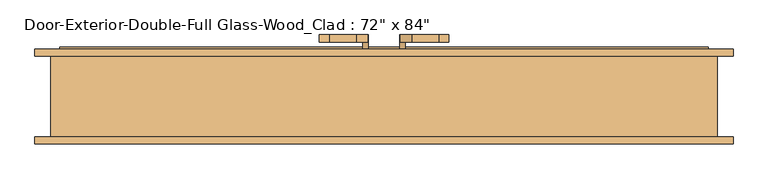
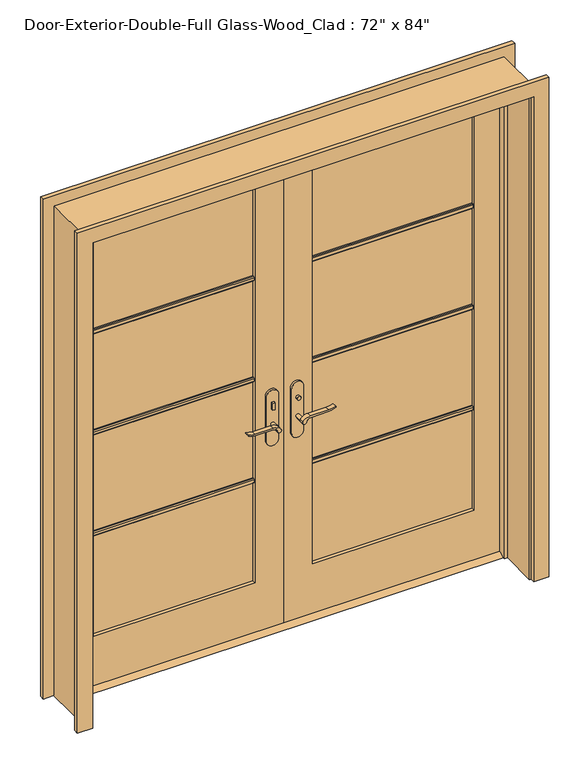
"""IFC4 building model written with IfcOpenShell, lengths in millimetres: door geometry."""

from ifc_helpers import new_model, si_unit, point, frame, frame_2d, origin, place, context, project, spatial, polyline, circle_curve, trimmed, segment, composite_curve, outline, extrude, faceted_brep, source, transform, mapped, element, save


def door_5bfea099(model_context):
    return source(origin(), model_context, "Body", "SolidModel", [
        extrude(outline(polyline([(76.2, 12.7), (111.125, 12.7), (136.525, 0.0), (50.8, 0.0), (76.2, 12.7)])), frame((-914.4, 0.0, 0.0), z_axis=(1.0, 0.0, 0.0), x_axis=(0.0, 1.0, 0.0)), (0.0, 0.0, 1.0), 1828.8),
        extrude(outline(polyline([(-47.4019111, 56.2), (-57.4019111, 56.2), (-57.4019111, 66.2), (-47.4019111, 66.2), (-47.4019111, 56.2)])), frame((0.0, 0.0, 981.9), z_axis=(0.0, 0.0, 1.0), x_axis=(1.0, 0.0, 0.0)), (0.0, 0.0, 1.0), 30.0),
        extrude(outline(composite_curve([segment(trimmed(circle_curve(frame_2d((996.9, -52.4019111)), 8.0), [point((996.9, -60.4019111))], [point((996.9, -44.4019111))], False, "CARTESIAN"), True, "CONTINUOUS"), segment(trimmed(circle_curve(frame_2d((996.9, -52.4019111)), 8.0), [point((996.9, -44.4019111))], [point((996.9, -60.4019111))], False, "CARTESIAN"), True, "CONTINUOUS")], self_intersect=False)), frame((0.0, 121.125, 0.0), z_axis=(0.0, 1.0, 0.0), x_axis=(0.0, 0.0, 1.0)), (0.0, 0.0, 1.0), 10.0),
        extrude(outline(composite_curve([segment(trimmed(circle_curve(frame_2d((897.1555521, -76.0694241)), 37.2832219), [point((919.0523287, -45.8937749))], [point((934.4, -77.7693445))], False, "CARTESIAN"), True, "CONTINUOUS"), segment(polyline([(934.4, -77.7693445), (934.4, -154.045502)]), True, "CONTINUOUS"), segment(trimmed(circle_curve(frame_2d((1017.6850638, -153.9791202)), 83.2850902), [point((934.4, -154.045502))], [point((939.4, -182.4019111))], True, "CARTESIAN"), True, "CONTINUOUS"), segment(polyline([(939.4, -182.4019111), (936.6135558, -182.4019111)]), True, "CONTINUOUS"), segment(trimmed(circle_curve(frame_2d((986.6709207, -150.4622499)), 59.3791355), [point((936.6135558, -182.4019111))], [point((927.4, -154.045502))], False, "CARTESIAN"), True, "CONTINUOUS"), segment(polyline([(927.4, -154.045502), (927.4, -77.7881013)]), True, "CONTINUOUS"), segment(trimmed(circle_curve(frame_2d((909.2738613, -77.7881013)), 18.1261387), [point((927.4, -77.7881013))], [point((914.4, -60.4019111))], True, "CARTESIAN"), True, "CONTINUOUS"), segment(trimmed(circle_curve(frame_2d((914.4, -52.4019111)), 8.0), [point((914.4, -60.4019111))], [point((919.0523287, -45.8937749))], False, "CARTESIAN"), True, "CONTINUOUS")], self_intersect=False)), frame((0.0, 16.2, 0.0), z_axis=(0.0, 1.0, 0.0), x_axis=(0.0, 0.0, 1.0)), (0.0, 0.0, 1.0), 20.0),
        extrude(outline(composite_curve([segment(trimmed(circle_curve(frame_2d((914.4, -52.4019111)), 8.0), [point((914.3999903, -60.4019111))], [point((919.0523287, -45.8937749))], False, "CARTESIAN"), True, "CONTINUOUS"), segment(trimmed(circle_curve(frame_2d((897.1555521, -76.0694241)), 37.2832219), [point((919.0523287, -45.8937749))], [point((934.4, -77.7693445))], False, "CARTESIAN"), True, "CONTINUOUS"), segment(polyline([(934.4, -77.7693445), (934.4, -154.045502)]), True, "CONTINUOUS"), segment(trimmed(circle_curve(frame_2d((1017.6850638, -153.9791202)), 83.2850902), [point((934.4, -154.045502))], [point((939.4, -182.4019111))], True, "CARTESIAN"), True, "CONTINUOUS"), segment(polyline([(939.4, -182.4019111), (936.6135558, -182.4019111)]), True, "CONTINUOUS"), segment(trimmed(circle_curve(frame_2d((986.6709207, -150.4622499)), 59.3791355), [point((936.6135558, -182.4019111))], [point((927.4, -154.045502))], False, "CARTESIAN"), True, "CONTINUOUS"), segment(polyline([(927.4, -154.045502), (927.4, -77.788099)]), True, "CONTINUOUS"), segment(trimmed(circle_curve(frame_2d((909.2738682, -77.788099)), 18.1261318), [point((927.4, -77.788099))], [point((914.3999903, -60.4019111))], True, "CARTESIAN"), True, "CONTINUOUS")], self_intersect=False)), frame((0.0, 151.125, 0.0), z_axis=(0.0, 1.0, 0.0), x_axis=(0.0, 0.0, 1.0)), (0.0, 0.0, 1.0), 20.0),
        extrude(outline(composite_curve([segment(trimmed(circle_curve(frame_2d((914.4, -52.4019111)), 8.0), [point((914.4, -60.4019111))], [point((914.4, -44.4019111))], False, "CARTESIAN"), True, "CONTINUOUS"), segment(trimmed(circle_curve(frame_2d((914.4, -52.4019111)), 8.0), [point((914.4, -44.4019111))], [point((914.4, -60.4019111))], False, "CARTESIAN"), True, "CONTINUOUS")], self_intersect=False)), frame((0.0, 36.2, 0.0), z_axis=(0.0, 1.0, 0.0), x_axis=(0.0, 0.0, 1.0)), (0.0, 0.0, 1.0), 30.0),
        extrude(outline(composite_curve([segment(trimmed(circle_curve(frame_2d((914.4, -52.4019111)), 8.0), [point((914.4, -60.4019111))], [point((914.4, -44.4019111))], False, "CARTESIAN"), True, "CONTINUOUS"), segment(trimmed(circle_curve(frame_2d((914.4, -52.4019111)), 8.0), [point((914.4, -44.4019111))], [point((914.4, -60.4019111))], False, "CARTESIAN"), True, "CONTINUOUS")], self_intersect=False)), frame((0.0, 121.125, 0.0), z_axis=(0.0, 1.0, 0.0), x_axis=(0.0, 0.0, 1.0)), (0.0, 0.0, 1.0), 30.0),
        extrude(outline(composite_curve([segment(polyline([(844.4, -27.4019111), (1039.4, -27.4019111)]), True, "CONTINUOUS"), segment(trimmed(circle_curve(frame_2d((1039.4, -52.4019111)), 25.0), [point((1039.4, -27.4019111))], [point((1039.4, -77.4019111))], False, "CARTESIAN"), True, "CONTINUOUS"), segment(polyline([(1039.4, -77.4019111), (844.4, -77.4019111)]), True, "CONTINUOUS"), segment(trimmed(circle_curve(frame_2d((844.4, -52.4019111)), 25.0), [point((844.4, -77.4019111))], [point((844.4, -27.4019111))], False, "CARTESIAN"), True, "CONTINUOUS")], self_intersect=False)), frame((0.0, 66.2, 0.0), z_axis=(0.0, 1.0, 0.0), x_axis=(0.0, 0.0, 1.0)), (0.0, 0.0, 1.0), 10.0),
        extrude(outline(composite_curve([segment(polyline([(844.4, -27.4019111), (1039.4, -27.4019111)]), True, "CONTINUOUS"), segment(trimmed(circle_curve(frame_2d((1039.4, -52.4019111)), 25.0), [point((1039.4, -27.4019111))], [point((1039.4, -77.4019111))], False, "CARTESIAN"), True, "CONTINUOUS"), segment(polyline([(1039.4, -77.4019111), (844.4, -77.4019111)]), True, "CONTINUOUS"), segment(trimmed(circle_curve(frame_2d((844.4, -52.4019111)), 25.0), [point((844.4, -77.4019111))], [point((844.4, -27.4019111))], False, "CARTESIAN"), True, "CONTINUOUS")], self_intersect=False)), frame((0.0, 111.125, 0.0), z_axis=(0.0, 1.0, 0.0), x_axis=(0.0, 0.0, 1.0)), (0.0, 0.0, 1.0), 10.0),
        extrude(outline(polyline([(47.3875, 131.125), (57.3875, 131.125), (57.3875, 121.125), (47.3875, 121.125), (47.3875, 131.125)])), frame((0.0, 0.0, 981.9), z_axis=(0.0, 0.0, 1.0), x_axis=(1.0, 0.0, 0.0)), (0.0, 0.0, 1.0), 30.0),
        extrude(outline(composite_curve([segment(trimmed(circle_curve(frame_2d((996.9, 52.3875)), 8.0), [point((996.9, 60.3875))], [point((996.9, 44.3875))], False, "CARTESIAN"), True, "CONTINUOUS"), segment(trimmed(circle_curve(frame_2d((996.9, 52.3875)), 8.0), [point((996.9, 44.3875))], [point((996.9, 60.3875))], False, "CARTESIAN"), True, "CONTINUOUS")], self_intersect=False)), frame((0.0, 56.2, 0.0), z_axis=(0.0, 1.0, 0.0), x_axis=(0.0, 0.0, 1.0)), (0.0, 0.0, 1.0), 10.0),
        extrude(outline(composite_curve([segment(trimmed(circle_curve(frame_2d((914.4, 52.3875)), 8.0), [point((919.0523287, 45.8793637))], [point((914.4, 60.3875))], False, "CARTESIAN"), True, "CONTINUOUS"), segment(trimmed(circle_curve(frame_2d((909.2738613, 77.7736901)), 18.1261387), [point((914.4, 60.3875))], [point((927.4, 77.7736901))], True, "CARTESIAN"), True, "CONTINUOUS"), segment(polyline([(927.4, 77.7736901), (927.4, 154.0310909)]), True, "CONTINUOUS"), segment(trimmed(circle_curve(frame_2d((986.6709207, 150.4478388)), 59.3791355), [point((927.4, 154.0310909))], [point((936.6135558, 182.3875))], False, "CARTESIAN"), True, "CONTINUOUS"), segment(polyline([(936.6135558, 182.3875), (939.4, 182.3875)]), True, "CONTINUOUS"), segment(trimmed(circle_curve(frame_2d((1017.6850638, 153.9647091)), 83.2850902), [point((939.4, 182.3875))], [point((934.4, 154.0310909))], True, "CARTESIAN"), True, "CONTINUOUS"), segment(polyline([(934.4, 154.0310909), (934.4, 77.7549333)]), True, "CONTINUOUS"), segment(trimmed(circle_curve(frame_2d((897.1555521, 76.0550129)), 37.2832219), [point((934.4, 77.7549333))], [point((919.0523287, 45.8793637))], False, "CARTESIAN"), True, "CONTINUOUS")], self_intersect=False)), frame((0.0, 151.125, 0.0), z_axis=(0.0, 1.0, 0.0), x_axis=(0.0, 0.0, 1.0)), (0.0, 0.0, 1.0), 20.0),
        extrude(outline(composite_curve([segment(trimmed(circle_curve(frame_2d((909.2738682, 77.7736878)), 18.1261318), [point((914.3999903, 60.3875))], [point((927.4, 77.7736878))], True, "CARTESIAN"), True, "CONTINUOUS"), segment(polyline([(927.4, 77.7736878), (927.4, 154.0310909)]), True, "CONTINUOUS"), segment(trimmed(circle_curve(frame_2d((986.6709207, 150.4478388)), 59.3791355), [point((927.4, 154.0310909))], [point((936.6135558, 182.3875))], False, "CARTESIAN"), True, "CONTINUOUS"), segment(polyline([(936.6135558, 182.3875), (939.4, 182.3875)]), True, "CONTINUOUS"), segment(trimmed(circle_curve(frame_2d((1017.6850638, 153.9647091)), 83.2850902), [point((939.4, 182.3875))], [point((934.4, 154.0310909))], True, "CARTESIAN"), True, "CONTINUOUS"), segment(polyline([(934.4, 154.0310909), (934.4, 77.7549333)]), True, "CONTINUOUS"), segment(trimmed(circle_curve(frame_2d((897.1555521, 76.0550129)), 37.2832219), [point((934.4, 77.7549333))], [point((919.0523287, 45.8793637))], False, "CARTESIAN"), True, "CONTINUOUS"), segment(trimmed(circle_curve(frame_2d((914.4, 52.3875)), 8.0), [point((919.0523287, 45.8793637))], [point((914.3999903, 60.3875))], False, "CARTESIAN"), True, "CONTINUOUS")], self_intersect=False)), frame((0.0, 16.2, 0.0), z_axis=(0.0, 1.0, 0.0), x_axis=(0.0, 0.0, 1.0)), (0.0, 0.0, 1.0), 20.0),
        extrude(outline(composite_curve([segment(trimmed(circle_curve(frame_2d((914.4, 52.3875)), 8.0), [point((914.4, 60.3875))], [point((914.4, 44.3875))], False, "CARTESIAN"), True, "CONTINUOUS"), segment(trimmed(circle_curve(frame_2d((914.4, 52.3875)), 8.0), [point((914.4, 44.3875))], [point((914.4, 60.3875))], False, "CARTESIAN"), True, "CONTINUOUS")], self_intersect=False)), frame((0.0, 121.125, 0.0), z_axis=(0.0, 1.0, 0.0), x_axis=(0.0, 0.0, 1.0)), (0.0, 0.0, 1.0), 30.0),
        extrude(outline(composite_curve([segment(trimmed(circle_curve(frame_2d((914.4, 52.3875)), 8.0), [point((914.4, 60.3875))], [point((914.4, 44.3875))], False, "CARTESIAN"), True, "CONTINUOUS"), segment(trimmed(circle_curve(frame_2d((914.4, 52.3875)), 8.0), [point((914.4, 44.3875))], [point((914.4, 60.3875))], False, "CARTESIAN"), True, "CONTINUOUS")], self_intersect=False)), frame((0.0, 36.2, 0.0), z_axis=(0.0, 1.0, 0.0), x_axis=(0.0, 0.0, 1.0)), (0.0, 0.0, 1.0), 30.0),
        extrude(outline(composite_curve([segment(trimmed(circle_curve(frame_2d((844.4, 52.3875)), 25.0), [point((844.4, 27.3875))], [point((844.4, 77.3875))], False, "CARTESIAN"), True, "CONTINUOUS"), segment(polyline([(844.4, 77.3875), (1039.4, 77.3875)]), True, "CONTINUOUS"), segment(trimmed(circle_curve(frame_2d((1039.4, 52.3875)), 25.0), [point((1039.4, 77.3875))], [point((1039.4, 27.3875))], False, "CARTESIAN"), True, "CONTINUOUS"), segment(polyline([(1039.4, 27.3875), (844.4, 27.3875)]), True, "CONTINUOUS")], self_intersect=False)), frame((0.0, 111.125, 0.0), z_axis=(0.0, 1.0, 0.0), x_axis=(0.0, 0.0, 1.0)), (0.0, 0.0, 1.0), 10.0),
        extrude(outline(composite_curve([segment(trimmed(circle_curve(frame_2d((844.4, 52.3875)), 25.0), [point((844.4, 27.3875))], [point((844.4, 77.3875))], False, "CARTESIAN"), True, "CONTINUOUS"), segment(polyline([(844.4, 77.3875), (1039.4, 77.3875)]), True, "CONTINUOUS"), segment(trimmed(circle_curve(frame_2d((1039.4, 52.3875)), 25.0), [point((1039.4, 77.3875))], [point((1039.4, 27.3875))], False, "CARTESIAN"), True, "CONTINUOUS"), segment(polyline([(1039.4, 27.3875), (844.4, 27.3875)]), True, "CONTINUOUS")], self_intersect=False)), frame((0.0, 66.2, 0.0), z_axis=(0.0, 1.0, 0.0), x_axis=(0.0, 0.0, 1.0)), (0.0, 0.0, 1.0), 10.0),
        extrude(outline(polyline([(90.17, 1578.371875), (90.17, 1559.321875), (83.82, 1559.321875), (80.645, 1562.496875), (80.645, 1575.196875), (83.82, 1578.371875), (90.17, 1578.371875)])), frame((120.65, 0.0, 0.0), z_axis=(1.0, 0.0, 0.0), x_axis=(0.0, 1.0, 0.0)), (0.0, 0.0, 1.0), 673.1),
        extrude(outline(polyline([(90.17, 1132.68125), (90.17, 1113.63125), (83.82, 1113.63125), (80.645, 1116.80625), (80.645, 1129.50625), (83.82, 1132.68125), (90.17, 1132.68125)])), frame((120.65, 0.0, 0.0), z_axis=(1.0, 0.0, 0.0), x_axis=(0.0, 1.0, 0.0)), (0.0, 0.0, 1.0), 673.1),
        extrude(outline(polyline([(90.17, 686.990625), (90.17, 667.940625), (83.82, 667.940625), (80.645, 671.115625), (80.645, 683.815625), (83.82, 686.990625), (90.17, 686.990625)])), frame((120.65, 0.0, 0.0), z_axis=(1.0, 0.0, 0.0), x_axis=(0.0, 1.0, 0.0)), (0.0, 0.0, 1.0), 673.1),
        extrude(outline(polyline([(97.155, 1578.371875), (103.505, 1578.371875), (106.68, 1575.196875), (106.68, 1562.496875), (103.505, 1559.321875), (97.155, 1559.321875), (97.155, 1578.371875)])), frame((-793.75, 0.0, 0.0), z_axis=(1.0, 0.0, 0.0), x_axis=(0.0, 1.0, 0.0)), (0.0, 0.0, 1.0), 673.1),
        extrude(outline(polyline([(97.155, 1132.68125), (103.505, 1132.68125), (106.68, 1129.50625), (106.68, 1116.80625), (103.505, 1113.63125), (97.155, 1113.63125), (97.155, 1132.68125)])), frame((-793.75, 0.0, 0.0), z_axis=(1.0, 0.0, 0.0), x_axis=(0.0, 1.0, 0.0)), (0.0, 0.0, 1.0), 673.1),
        extrude(outline(polyline([(97.155, 686.990625), (103.505, 686.990625), (106.68, 683.815625), (106.68, 671.115625), (103.505, 667.940625), (97.155, 667.940625), (97.155, 686.990625)])), frame((-793.75, 0.0, 0.0), z_axis=(1.0, 0.0, 0.0), x_axis=(0.0, 1.0, 0.0)), (0.0, 0.0, 1.0), 673.1),
        extrude(outline(polyline([(97.155, 1578.371875), (103.505, 1578.371875), (106.68, 1575.196875), (106.68, 1562.496875), (103.505, 1559.321875), (97.155, 1559.321875), (97.155, 1578.371875)])), frame((120.65, 0.0, 0.0), z_axis=(1.0, 0.0, 0.0), x_axis=(0.0, 1.0, 0.0)), (0.0, 0.0, 1.0), 673.1),
        extrude(outline(polyline([(97.155, 1132.68125), (103.505, 1132.68125), (106.68, 1129.50625), (106.68, 1116.80625), (103.505, 1113.63125), (97.155, 1113.63125), (97.155, 1132.68125)])), frame((120.65, 0.0, 0.0), z_axis=(1.0, 0.0, 0.0), x_axis=(0.0, 1.0, 0.0)), (0.0, 0.0, 1.0), 673.1),
        extrude(outline(polyline([(97.155, 686.990625), (103.505, 686.990625), (106.68, 683.815625), (106.68, 671.115625), (103.505, 667.940625), (97.155, 667.940625), (97.155, 686.990625)])), frame((120.65, 0.0, 0.0), z_axis=(1.0, 0.0, 0.0), x_axis=(0.0, 1.0, 0.0)), (0.0, 0.0, 1.0), 673.1),
        extrude(outline(polyline([(90.17, 1578.371875), (90.17, 1559.321875), (83.82, 1559.321875), (80.645, 1562.496875), (80.645, 1575.196875), (83.82, 1578.371875), (90.17, 1578.371875)])), frame((-793.75, 0.0, 0.0), z_axis=(1.0, 0.0, 0.0), x_axis=(0.0, 1.0, 0.0)), (0.0, 0.0, 1.0), 673.1),
        extrude(outline(polyline([(90.17, 1132.68125), (90.17, 1113.63125), (83.82, 1113.63125), (80.645, 1116.80625), (80.645, 1129.50625), (83.82, 1132.68125), (90.17, 1132.68125)])), frame((-793.75, 0.0, 0.0), z_axis=(1.0, 0.0, 0.0), x_axis=(0.0, 1.0, 0.0)), (0.0, 0.0, 1.0), 673.1),
        extrude(outline(polyline([(90.17, 686.990625), (90.17, 667.940625), (83.82, 667.940625), (80.645, 671.115625), (80.645, 683.815625), (83.82, 686.990625), (90.17, 686.990625)])), frame((-793.75, 0.0, 0.0), z_axis=(1.0, 0.0, 0.0), x_axis=(0.0, 1.0, 0.0)), (0.0, 0.0, 1.0), 673.1),
        extrude(outline(polyline([(0.0, 920.75), (0.0, 984.25), (2203.45, 984.25), (2203.45, -984.25), (0.0, -984.25), (0.0, -920.75), (2139.95, -920.75), (2139.95, 920.75), (0.0, 920.75)])), frame((0.0, 111.125, 0.0), z_axis=(0.0, 1.0, 0.0), x_axis=(0.0, 0.0, 1.0)), (0.0, 0.0, 1.0), 19.05),
        extrude(outline(polyline([(0.0, 920.75), (0.0, 984.25), (2203.45, 984.25), (2203.45, -984.25), (0.0, -984.25), (0.0, -920.75), (2139.95, -920.75), (2139.95, 920.75), (0.0, 920.75)])), frame((0.0, -136.525, 0.0), z_axis=(0.0, 1.0, 0.0), x_axis=(0.0, 0.0, 1.0)), (0.0, 0.0, 1.0), 19.05),
        extrude(outline(polyline([(12.7, 914.4), (2133.6, 914.4), (2133.6, 1.5875), (12.7, 1.5875), (12.7, 914.4)]), holes=[polyline([(2014.5375, 120.65), (2014.5375, 793.75), (231.775, 793.75), (231.775, 120.65), (2014.5375, 120.65)])]), frame((0.0, 76.2, 0.0), z_axis=(0.0, 1.0, 0.0), x_axis=(0.0, 0.0, 1.0)), (0.0, 0.0, 1.0), 34.925),
        extrude(outline(polyline([(2133.6, -914.4), (12.7, -914.4), (12.7, -1.6019111), (2133.6, -1.6019111), (2133.6, -914.4)]), holes=[polyline([(231.775, -793.75), (2014.5375, -793.75), (2014.5375, -120.65), (231.775, -120.65), (231.775, -793.75)])]), frame((0.0, 76.2, 0.0), z_axis=(0.0, 1.0, 0.0), x_axis=(0.0, 0.0, 1.0)), (0.0, 0.0, 1.0), 34.925),
        faceted_brep([(939.8, 111.125, 0.0), (939.8, -117.475, 0.0), (914.4, -117.475, 0.0), (914.4, 41.275, 0.0), (901.7, 41.275, 0.0), (901.7, 76.2, 0.0), (914.4, 76.2, 0.0), (914.4, 111.125, 0.0), (939.8, 111.125, 2159.0), (939.8, -117.475, 2159.0), (-939.8, -117.475, 2159.0), (-939.8, -117.475, 0.0), (-914.4, -117.475, 0.0), (-914.4, -117.475, 2133.6), (914.4, -117.475, 2133.6), (914.4, 41.275, 2133.6), (-914.4, 41.275, 2133.6), (-914.4, 41.275, 0.0), (-901.7, 41.275, 0.0), (-901.7, 41.275, 2120.9), (901.7, 41.275, 2120.9), (901.7, 76.2, 2120.9), (1.5875, 76.2, 2120.9), (-1.6019111, 76.2, 2120.9), (-901.7, 76.2, 2120.9), (-901.7, 76.2, 0.0), (-914.4, 76.2, 0.0), (-914.4, 76.2, 2133.6), (-1.6019111, 76.2, 2133.6), (1.5875, 76.2, 2133.6), (914.4, 76.2, 2133.6), (914.4, 111.125, 2133.6), (1.5875, 111.125, 2133.6), (-1.6019111, 111.125, 2133.6), (-914.4, 111.125, 2133.6), (-914.4, 111.125, 0.0), (-939.8, 111.125, 0.0), (-939.8, 111.125, 2159.0)], [[[0, 1, 2, 3, 4, 5, 6, 7]], [[1, 0, 8, 9]], [[2, 1, 9, 10, 11, 12, 13, 14]], [[3, 2, 14, 15]], [[4, 3, 15, 16, 17, 18, 19, 20]], [[5, 4, 20, 21]], [[6, 5, 21, 22, 23, 24, 25, 26, 27, 28, 29, 30]], [[7, 6, 30, 31]], [[0, 7, 31, 32, 33, 34, 35, 36, 37, 8]], [[9, 8, 37, 10]], [[14, 13, 16, 15]], [[20, 19, 24, 23, 22, 21]], [[31, 30, 29, 28, 27, 34, 33, 32]], [[12, 11, 36, 35, 26, 25, 18, 17]], [[11, 10, 37, 36]], [[13, 12, 17, 16]], [[19, 18, 25, 24]], [[27, 26, 35, 34]]]),
        extrude(outline(polyline([(793.75, 90.17), (120.65, 90.17), (120.65, 97.155), (793.75, 97.155), (793.75, 90.17)])), frame((0.0, 0.0, 231.775), z_axis=(0.0, 0.0, 1.0), x_axis=(1.0, 0.0, 0.0)), (0.0, 0.0, 1.0), 1782.7625),
        extrude(outline(polyline([(-120.65, 90.17), (-793.75, 90.17), (-793.75, 97.155), (-120.65, 97.155), (-120.65, 90.17)])), frame((0.0, 0.0, 231.775), z_axis=(0.0, 0.0, 1.0), x_axis=(1.0, 0.0, 0.0)), (0.0, 0.0, 1.0), 1782.7625),
    ])


if __name__ == "__main__":
    model = new_model("IFC4")
    model_context = context("Model", 3, world=origin())
    ifc_project = project(units=[si_unit("LENGTHUNIT", "METRE", prefix="MILLI")], contexts=[model_context])
    site = spatial("IfcSite", under=ifc_project)
    building = spatial("IfcBuilding", under=site)
    placement = place(None, origin())
    door_shape = door_5bfea099(model_context)
    element("IfcDoor", 1, ObjectType="Door-Exterior-Double-Full Glass-Wood_Clad : 72\" x 84\"", at=placement, inside=building, context=model_context, shape_type="MappedRepresentation", body=[
        mapped(door_shape, transform((0.0, 0.0, 0.0), x_axis=(1.0, 0.0, 0.0), y_axis=(0.0, 1.0, 0.0), z_axis=(0.0, 0.0, 1.0))),
    ])
    save(model, "model.ifc")

# Revit data of these elements
# Type "Door-Exterior-Double-Full Glass-Wood_Clad : 72\" x 84\""
#   Type Mark = "10"
#   Assembly Code = "B2030100"
#   Analytic Construction = "French door, wood frame with double glass"
#   Top Rail = 0' - 4 11/16"
#   Threshold Offset [instance default] = 0' - 0 1/2"
#   Thickness = 0' - 1 3/8"
#   Thermal Resistance (R) = 1.9158 (h·ft²·°F)/BTU
#   Swing Angle [instance default] = 90.00°
#   Stiles = 0' - 4 3/4"
#   Rough Width = 6' - 2"
#   Rough Height = 7' - 1"
#   Panel Width = 3' - 0"
#   Door Offset [instance default] = 0' - 0"
#   Height = 7' - 0"
#   Width = 6' - 0"
#   Heat Transfer Coefficient (U) = 0.5220 BTU/(h·ft²·°F)
#   Bottom Rail = 0' - 9 1/8"
#   Exterior Trim [instance default] = yes
#   Threshold [instance default] = yes
#   Show Grill [instance default] = yes
#   Function = 1
#   Trim Material = Cherry
#   Threshold Material = Cherry
#   Panel Material = Cherry
#   Glazing = Glass
#   Frame Material = Cherry
#   Door Handle Material = Aluminum
#   Visual Light Transmittance = 0
#   Solar Heat Gain Coefficient = 0
#   Wall Closure = (empty or 0)
#   Construction Type = (empty or 0)
# Element 1 (IfcDoor, "Door-Exterior-Double-Full Glass-Wood_Clad : 72\" x 84\"")
#   Materials on its faces: "Cherry", "Aluminum", "Glass"
# Materials
#   "Cherry": class "Wood", colour RGB 226 177 128, transparency 0, Description = "Prunus Serotina", Cost = 0
#   "Glass": class "Glass", colour RGB 0 128 192, transparency 0.75, Description = "Soda Lime Glass", Cost = 0
#   "Aluminum": class "Metal", colour RGB 247 247 247, transparency 0, Description = "Aluminum 6061", Cost = 0
